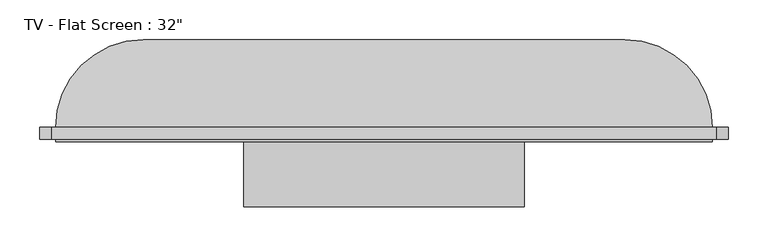
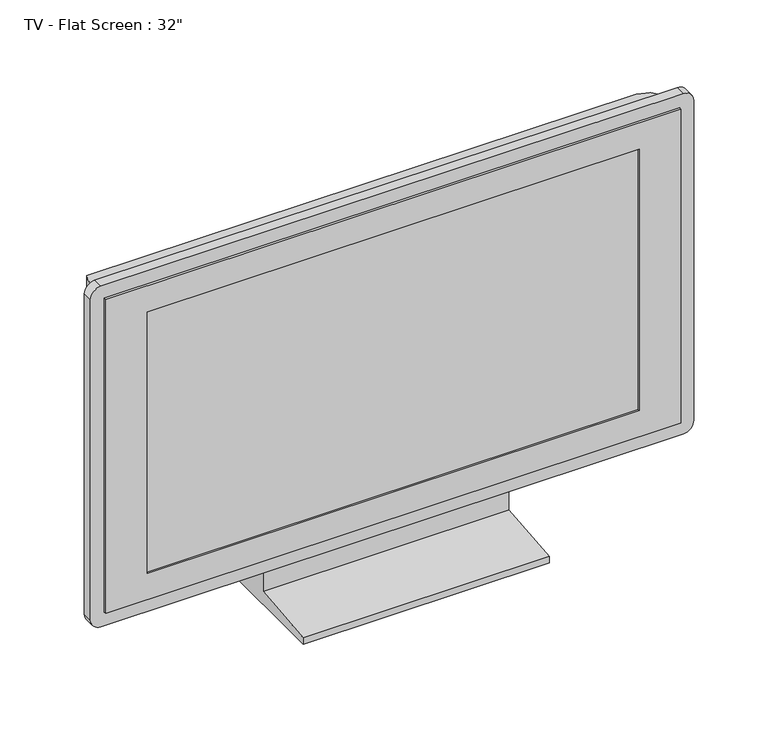
"""IFC4 building model written with IfcOpenShell, lengths in millimetres: furniture geometry."""

from ifc_helpers import new_model, si_unit, point, frame, frame_2d, origin, place, context, project, spatial, polyline, circle_curve, ellipse_curve, trimmed, segment, composite_curve, outline, extrude, faceted_brep, source, transform, mapped, element, save
from ifc_brep_helpers import plane_surface, cylinder_surface, advanced_brep


def furniture_51289c3c(model_context):
    return source(origin(), model_context, "Body", "SolidModel", [
        advanced_brep(
        [(-416.9248214, -51.4613764, 80.0), (409.0357931, -51.4613764, 80.0), (409.0357931, -51.4613764, 557.1392838), (-416.9248214, -51.4613764, 557.1392838), (299.0357931, 58.5386236, 80.0), (-306.9248214, 58.5386236, 80.0), (-306.9248214, 58.5386236, 447.1392838), (299.0357931, 58.5386236, 447.1392838)],
        [
            (0, 1),
            (1, 2),
            (2, 3),
            (3, 0),
            (4, 5),
            (5, 6),
            (6, 7),
            (7, 4),
            (0, 5, circle_curve(frame((-306.9248214, -51.4613764, 80.0), z_axis=(0.0, 0.0, -1.0), x_axis=(-1.0, 0.0, 0.0)), 110.0)),
            (4, 1, circle_curve(frame((299.0357931, -51.4613764, 80.0), z_axis=(0.0, 0.0, -1.0), x_axis=(1.0, 0.0, 0.0)), 110.0)),
            (7, 2, ellipse_curve(frame((299.0357931, -51.4613764, 447.1392838), z_axis=(0.7071067811865475, 0.0, -0.7071067811865475), x_axis=(0.7071067811865474, 0.0, 0.7071067811865476)), 155.5634919, 110.0)),
            (6, 3, ellipse_curve(frame((-306.9248214, -51.4613764, 447.1392838), z_axis=(0.7071067811865475, 0.0, 0.7071067811865475), x_axis=(-0.7071067811865476, 0.0, 0.7071067811865474)), 155.5634919, 110.0)),
        ],
        [
            plane_surface(frame((-416.9248214, -51.4613764, 557.1392838), z_axis=(0.0, -1.0, 0.0), x_axis=(-1.0, 0.0, 0.0))),
            plane_surface(frame((-416.9248214, 58.5386236, 557.1392838), z_axis=(0.0, 1.0, 0.0), x_axis=(1.0, 0.0, 0.0))),
            plane_surface(frame((-416.9248214, -51.4613764, 80.0), z_axis=(0.0, 0.0, -1.0), x_axis=(0.0, 1.0, 0.0))),
            cylinder_surface(frame((299.0357931, -51.4613764, 80.0), z_axis=(0.0, 0.0, 1.0), x_axis=(1.0, 0.0, 0.0)), 110.0),
            cylinder_surface(frame((409.0357931, -51.4613764, 447.1392838), z_axis=(-1.0, 0.0, 0.0), x_axis=(0.0, 0.0, 1.0)), 110.0),
            cylinder_surface(frame((-306.9248214, -51.4613764, 557.1392838), z_axis=(0.0, 0.0, -1.0), x_axis=(-1.0, 0.0, 0.0)), 110.0),
        ],
        [
            (0, [[1, 2, 3, 4]]),
            (1, [[5, 6, 7, 8]]),
            (2, [[-1, 9, -5, 10]]),
            (3, [[11, -2, -10, -8]]),
            (4, [[-11, -7, 12, -3]]),
            (5, [[-12, -6, -9, -4]]),
        ],
    ),
        extrude(outline(composite_curve([segment(polyline([(577.1392838, 414.0357931), (577.1392838, -421.9248214)]), True, "CONTINUOUS"), segment(trimmed(circle_curve(frame_2d((562.1392838, -421.9248214)), 15.0), [point((577.1392838, -421.9248214))], [point((562.1392838, -436.9248214))], False, "CARTESIAN"), True, "CONTINUOUS"), segment(polyline([(562.1392838, -436.9248214), (75.0, -436.9248214)]), True, "CONTINUOUS"), segment(trimmed(circle_curve(frame_2d((75.0, -421.9248214)), 15.0), [point((75.0, -436.9248214))], [point((60.0, -421.9248214))], False, "CARTESIAN"), True, "CONTINUOUS"), segment(polyline([(60.0, -421.9248214), (60.0, 414.0357931)]), True, "CONTINUOUS"), segment(trimmed(circle_curve(frame_2d((75.0, 414.0357931)), 15.0), [point((60.0, 414.0357931))], [point((75.0, 429.0357931))], False, "CARTESIAN"), True, "CONTINUOUS"), segment(polyline([(75.0, 429.0357931), (562.1392838, 429.0357931)]), True, "CONTINUOUS"), segment(trimmed(circle_curve(frame_2d((562.1392838, 414.0357931)), 15.0), [point((562.1392838, 429.0357931))], [point((577.1392838, 414.0357931))], False, "CARTESIAN"), True, "CONTINUOUS")], self_intersect=False), holes=[polyline([(557.1392838, 409.0357931), (80.0, 409.0357931), (80.0, -416.9248214), (557.1392838, -416.9248214), (557.1392838, 409.0357931)])]), frame((0.0, -66.4613764, 0.0), z_axis=(0.0, 1.0, 0.0), x_axis=(0.0, 0.0, 1.0)), (0.0, 0.0, 1.0), 15.0),
        faceted_brep([(409.0357931, -69.4613764, 557.1392838), (-416.9248214, -69.4613764, 557.1392838), (-416.9248214, -69.4613764, 80.0), (409.0357931, -69.4613764, 80.0), (-356.9248214, -69.4613764, 517.1392838), (349.0357931, -69.4613764, 517.1392838), (349.0357931, -69.4613764, 120.0), (-356.9248214, -69.4613764, 120.0), (409.0357931, -51.4613764, 557.1392838), (409.0357931, -51.4613764, 80.0), (-416.9248214, -51.4613764, 80.0), (-416.9248214, -51.4613764, 557.1392838), (-356.9248214, -66.4613764, 517.1392838), (-356.9248214, -66.4613764, 120.0), (349.0357931, -66.4613764, 120.0), (349.0357931, -66.4613764, 517.1392838)], [[[0, 1, 2, 3], [4, 5, 6, 7]], [[8, 9, 10, 11]], [[1, 0, 8, 11]], [[2, 1, 11, 10]], [[3, 2, 10, 9]], [[0, 3, 9, 8]], [[12, 13, 14, 15]], [[12, 15, 5, 4]], [[15, 14, 6, 5]], [[14, 13, 7, 6]], [[13, 12, 4, 7]]]),
        extrude(outline(polyline([(-51.4613764, 80.0), (-1.4613764, 80.0), (48.5386236, 0.0), (-151.4613764, 0.0), (-151.4613764, 10.0), (-51.4613764, 20.0), (-51.4613764, 80.0)])), frame((-180.4346678, 0.0, 0.0), z_axis=(1.0, 0.0, 0.0), x_axis=(0.0, 1.0, 0.0)), (0.0, 0.0, 1.0), 352.9803073),
    ])


if __name__ == "__main__":
    model = new_model("IFC4")
    model_context = context("Model", 3, world=origin())
    ifc_project = project(units=[si_unit("LENGTHUNIT", "METRE", prefix="MILLI")], contexts=[model_context])
    site = spatial("IfcSite", under=ifc_project)
    building = spatial("IfcBuilding", under=site)
    placement = place(None, origin())
    furniture_shape = furniture_51289c3c(model_context)
    element("IfcFurniture", 1, ObjectType="TV - Flat Screen : 32\"", at=placement, inside=building, context=model_context, shape_type="MappedRepresentation", body=[
        mapped(furniture_shape, transform((0.0, 0.0, 0.0), x_axis=(1.0, 0.0, 0.0), y_axis=(0.0, 1.0, 0.0), z_axis=(0.0, 0.0, 1.0))),
    ])
    save(model, "model.ifc")

# Revit data of these elements
# Type "TV - Flat Screen : 32\""
#   SinAng = 0.49 mm
#   L = 705.961 mm
#   H = 397.139 mm
#   Thickness = 110 mm
#   Diagonal = 810 mm
#   CosAng = 0.872 mm
#   Stand [instance default] = yes
#   Default Elevation = 0
# Element 1 (IfcFurniture, "TV - Flat Screen : 32\"")
#   Materials on its faces: "TV - Black", "TV - Glass", "TV - Screen"
# Materials
#   "TV - Black": colour RGB 49 49 49, transparency 0
#   "TV - Glass": colour RGB 157 157 157, transparency 0.9
#   "TV - Screen": colour RGB 0 0 0, transparency 0
